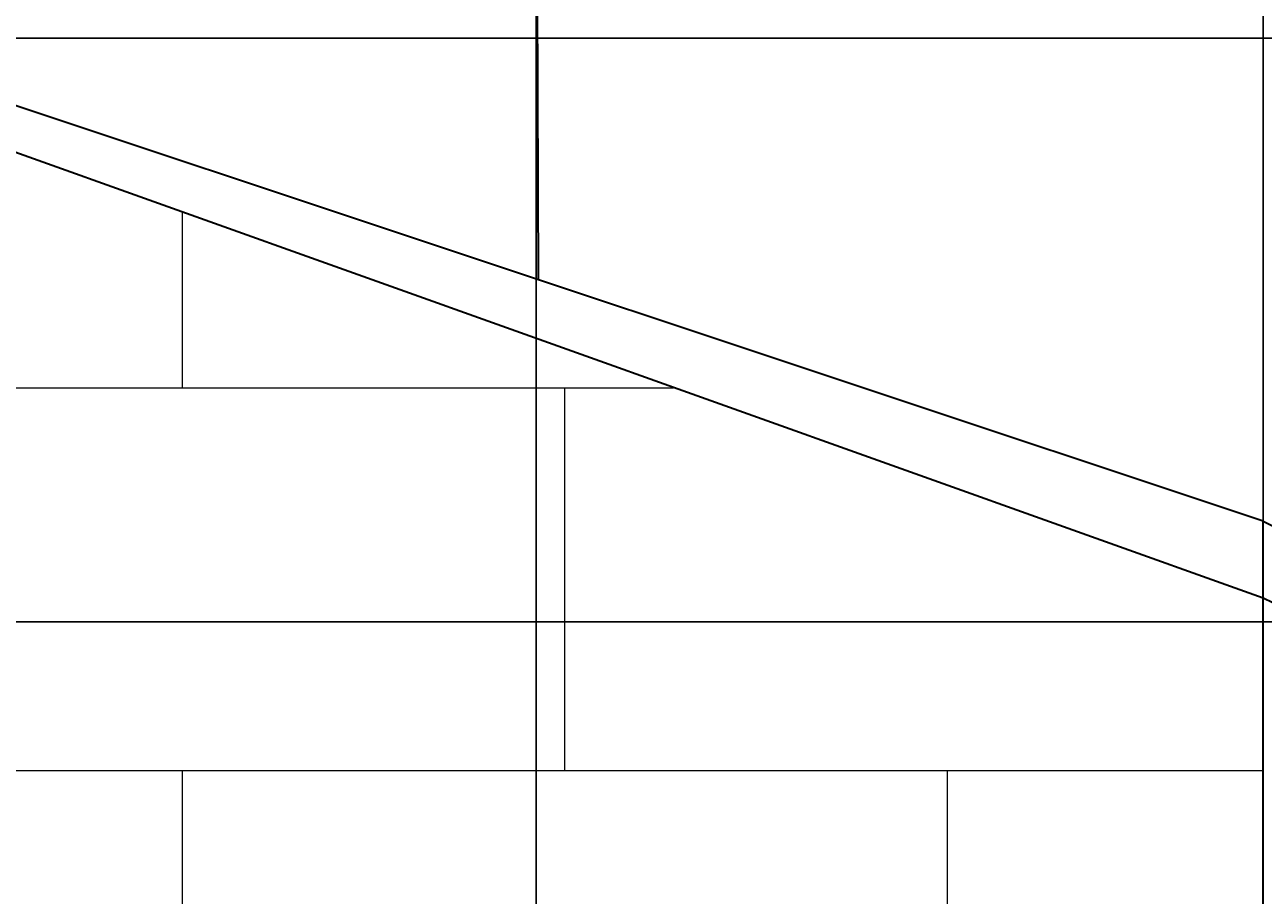
# Model space of a CAD drawing. Units: inches. Extents: x -26 to 776, y -22 to 650.
# Tile 38 of 62: x 309 to 426, y 420 to 502. Entities that reach past the tile are written whole.
import ezdxf

# ---------------------------------------------------------------- set-up
doc = ezdxf.new("R2010")
doc.units = ezdxf.units.IN
doc.header["$MEASUREMENT"] = 0
for name, color, linetype, lineweight in [('A-ANNO-DIMS', 2, 'Continuous', 18), ('A-ROOF', 7, 'Continuous', 35), ('A-WALL', 7, 'Continuous', 35), ('A-WALL-PATT', 8, 'Continuous', 13)]:
    doc.layers.add(name, color=color, linetype=linetype, lineweight=lineweight)
doc.styles.get("Standard").update_dxf_attribs({"font": 'arial.ttf'})
doc.dimstyles.get("Standard").update_dxf_attribs({"dimtxt": 0.5625, "dimasz": 0.18, "dimexe": 0.18, "dimexo": 0.0625, "dimgap": 0.09, "dimtad": 0, "dimtih": 1, "dimtoh": 1, "dimdec": 4, "dimzin": 0, "dimdsep": 46, "dimlunit": 4, "dimtxsty": 'Standard', "dimcen": 0.09, "dimadec": 0, "dimazin": 0, "dimtfac": 1, "dimtdec": 4, "dimtofl": 0, "dimtmove": 0, "dimatfit": 3, "dimfxl": 1, "dimtolj": 1, "dimtzin": 0, "dimarcsym": 0})

# ---------------------------------------------------------------- blocks, each defined once
blk = doc.blocks.new('*D9')
at = {"layer": 'A-ANNO-DIMS', "color": 0, "lineweight": -2, "transparency": 16777216}
for p, q in [((285.08, 446.01), (304.98, 446.01)), ((304.8, 445.83), (304.8, 380.44)), ((304.8, 314.3), (304.8, 379.68)), ((285.08, 314.12), (304.98, 314.12))]:
    blk.add_line(p, q, dxfattribs=at)
at = {"layer": 'A-ANNO-DIMS', "color": 0, "transparency": 16777216}
for points in [[(304.77, 445.83), (304.83, 445.83), (304.8, 446.01)], [(304.77, 314.3), (304.83, 314.3), (304.8, 314.12)]]:
    blk.add_solid(points, dxfattribs=at)
at = {"layer": 'Defpoints', "color": 0, "transparency": 16777216}
for p in [(285.02, 446.01), (304.8, 446.01), (285.02, 314.12)]:
    blk.add_point(p, dxfattribs=at)
at = {"layer": 'A-ANNO-DIMS', "color": 0, "transparency": 16777216, "insert": (304.8, 380.06), "char_height": 0.5625, "attachment_point": 5}
blk.add_mtext('\\A1;NARROW WINDOW 132 TYP.', dxfattribs=at)
blk = doc.blocks.new('*D31')
at = {"layer": 'A-ANNO-DIMS', "color": 0, "lineweight": -2, "transparency": 16777216}
for p, q in [((289.3, 500.9), (775.34, 500.9)), ((775.16, 500.72), (775.16, 473.83)), ((775.16, 446.19), (775.16, 473.07)), ((285.08, 446.01), (775.34, 446.01))]:
    blk.add_line(p, q, dxfattribs=at)
at = {"layer": 'A-ANNO-DIMS', "color": 0, "transparency": 16777216}
for points in [[(775.13, 500.72), (775.19, 500.72), (775.16, 500.9)], [(775.13, 446.19), (775.19, 446.19), (775.16, 446.01)]]:
    blk.add_solid(points, dxfattribs=at)
at = {"layer": 'Defpoints', "color": 0, "transparency": 16777216}
for p in [(289.24, 500.9), (775.16, 500.9), (285.02, 446.01)]:
    blk.add_point(p, dxfattribs=at)
at = {"layer": 'A-ANNO-DIMS', "color": 0, "transparency": 16777216, "insert": (775.16, 473.45), "char_height": 0.562, "attachment_point": 5}
blk.add_mtext('\\A1;54.89', dxfattribs=at)
blk = doc.blocks.new('*D34')
at = {"layer": 'A-ANNO-DIMS', "color": 0, "lineweight": -2, "transparency": 16777216}
for p, q in [((228.57, 528.3), (228.57, -21.31)), ((357.3, 528.36), (357.3, -21.31)), ((228.75, -21.13), (291.71, -21.13)), ((357.12, -21.13), (294.17, -21.13))]:
    blk.add_line(p, q, dxfattribs=at)
at = {"layer": 'A-ANNO-DIMS', "color": 0, "transparency": 16777216}
for points in [[(228.75, -21.1), (228.75, -21.16), (228.57, -21.13)], [(357.12, -21.1), (357.12, -21.16), (357.3, -21.13)]]:
    blk.add_solid(points, dxfattribs=at)
at = {"layer": 'Defpoints', "color": 0, "transparency": 16777216}
for p in [(228.57, 528.36), (357.3, 528.42), (357.3, -21.13)]:
    blk.add_point(p, dxfattribs=at)
at = {"layer": 'A-ANNO-DIMS', "color": 0, "transparency": 16777216, "insert": (292.94, -21.13), "char_height": 0.562, "attachment_point": 5}
blk.add_mtext('\\A1;128.73', dxfattribs=at)
blk = doc.blocks.new('*D39')
at = {"layer": 'A-ANNO-DIMS', "color": 0, "lineweight": -2, "transparency": 16777216}
for p, q in [((289.24, 15.54), (289.24, 649.86)), ((289.42, 649.68), (356.48, 649.68)), ((425.56, 649.68), (358.51, 649.68)), ((425.74, 15.54), (425.74, 649.86))]:
    blk.add_line(p, q, dxfattribs=at)
at = {"layer": 'A-ANNO-DIMS', "color": 0, "transparency": 16777216}
for points in [[(289.42, 649.71), (289.42, 649.65), (289.24, 649.68)], [(425.56, 649.71), (425.56, 649.65), (425.74, 649.68)]]:
    blk.add_solid(points, dxfattribs=at)
at = {"layer": 'Defpoints', "color": 0, "transparency": 16777216}
for p in [(425.74, 649.68), (289.24, 15.48), (425.74, 15.48)]:
    blk.add_point(p, dxfattribs=at)
at = {"layer": 'A-ANNO-DIMS', "color": 0, "transparency": 16777216, "insert": (357.49, 649.68), "char_height": 0.562, "attachment_point": 5}
blk.add_mtext('\\A1;136.5', dxfattribs=at)

msp = doc.modelspace()

# ---------------------------------------------------------------- hatches: boundary and pattern name
at = {"layer": 'A-WALL-PATT'}
h = msp.add_hatch(dxfattribs=at)
h.set_pattern_fill('AR-B816', color=256, scale=4.5)
h.paths.add_polyline_path([(425.7434, 448.2114), (289.2424, 496.9554), (289.2424, 458.1203), (289.2424, 291.1798), (289.2424, 20.7937), (425.7434, 20.7937), (425.7434, 283.2492)])

# ---------------------------------------------------------------- linework, layer by layer
at = {"layer": 'A-ROOF'}
for p, q in [((425.7434, 455.4717), (289.2424, 500.896)), ((425.7434, 448.2114), (289.2424, 496.9554)), ((425.7434, 455.4717), (448.0125, 444.3909)), ((444.9683, 438.8738), (425.7434, 448.2114))]:
    msp.add_line(p, q, dxfattribs=at)
at = {"layer": 'A-WALL'}
for p, q in [((357.0669, 613.2713), (357.4929, 478.1838)), ((425.7434, 283.2492), (425.7434, 455.4717))]:
    msp.add_line(p, q, dxfattribs=at)

# ---------------------------------------------------------------- dimensions: what is measured, and where the dimension line sits
at = {"layer": 'A-ANNO-DIMS'}
for base, p1, p2, override, picture, middle in [((425.7434, 649.6763), (289.2424, 15.4824), (425.7434, 15.4824), {"dimdec": 1, "dimlfac": 1, "dimrnd": 0, "dimzin": 0, "dimdsep": 46, "dimlunit": 2}, '*D39', (357.4929, 649.6763)), ((357.3034, -21.1349), (228.5733, 528.3585), (357.3034, 528.4233), {"dimdec": 2, "dimlfac": 1, "dimrnd": 0, "dimzin": 0, "dimdsep": 46, "dimlunit": 2}, '*D34', (292.9384, -21.1349))]:
    dim = msp.add_linear_dim(base=base, p1=p1, p2=p2, dimstyle='Standard', override=override, dxfattribs=at)
    dim.commit()
    dim.dimension.update_dxf_attribs({"geometry": picture, "text_midpoint": middle})
dim = msp.add_linear_dim(base=(775.1553, 500.896), p1=(285.0179, 446.0063), p2=(289.2424, 500.896), angle=90, dimstyle='Standard', override={"dimdec": 2, "dimlfac": 1, "dimrnd": 0, "dimzin": 0, "dimdsep": 46, "dimlunit": 2}, dxfattribs=at)
dim.commit()
dim.dimension.update_dxf_attribs({"geometry": '*D31', "text_midpoint": (775.1553, 473.4511)})
dim = msp.add_linear_dim(base=(304.801, 446.0063), p1=(285.0179, 314.119), p2=(285.0179, 446.0063), angle=90, text='NARROW WINDOW <> TYP.', dimstyle='Standard', override={"dimdec": 0, "dimlfac": 1, "dimrnd": 0, "dimzin": 0, "dimdsep": 46, "dimlunit": 2}, dxfattribs=at)
dim.commit()
dim.dimension.update_dxf_attribs({"geometry": '*D9', "text_midpoint": (304.801, 380.0626)})

doc.saveas('drawing.dxf')
